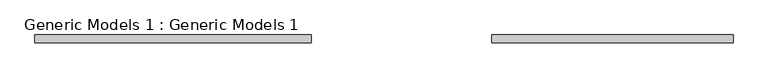
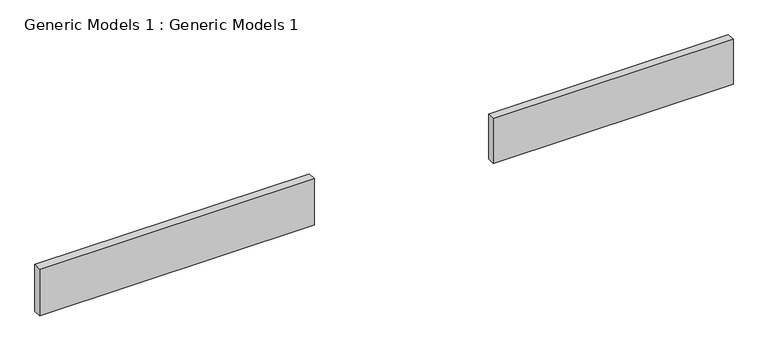
"""IFC4 building model written with IfcOpenShell, lengths in millimetres: proxy geometry, Generic Models 1 : Generic Models 1."""

from ifc_helpers import new_model, si_unit, frame, origin, place, context, project, spatial, polyline, outline, extrude, source, transform, mapped, element, save


def generic_models_1_generic_models_1_e0ba6133(model_context):
    return source(origin(), model_context, "Body", "SweptSolid", [
        extrude(outline(polyline([(5733.7651683, -9812.6503266), (1161.7651683, -9812.6503266), (1161.7651683, -9660.2503266), (5733.7651683, -9660.2503266), (5733.7651683, -9812.6503266)])), frame((0.0, 0.0, 357.9881609), z_axis=(0.0, 0.0, 1.0), x_axis=(1.0, 0.0, 0.0)), (0.0, 0.0, 1.0), 901.097394),
        extrude(outline(polyline([(-2253.6679045, -9812.6503266), (-7486.0679045, -9812.6503266), (-7486.0679045, -9660.2503266), (-2253.6679045, -9660.2503266), (-2253.6679045, -9812.6503266)])), frame((0.0, 0.0, 312.1459104), z_axis=(0.0, 0.0, 1.0), x_axis=(1.0, 0.0, 0.0)), (0.0, 0.0, 1.0), 939.8),
    ])


if __name__ == "__main__":
    model = new_model("IFC4")
    model_context = context("Model", 3, world=origin())
    ifc_project = project(units=[si_unit("LENGTHUNIT", "METRE", prefix="MILLI")], contexts=[model_context])
    site = spatial("IfcSite", under=ifc_project)
    building = spatial("IfcBuilding", under=site)
    placement = place(None, origin())
    generic_models_1_generic_models_1_shape = generic_models_1_generic_models_1_e0ba6133(model_context)
    element("IfcBuildingElementProxy", 1, Name="Generic Models 1 : Generic Models 1", ObjectType="Generic Models 1 : Generic Models 1", at=placement, inside=building, context=model_context, shape_type="MappedRepresentation", body=[
        mapped(generic_models_1_generic_models_1_shape, transform((0.0, 0.0, 0.0), x_axis=(1.0, 0.0, 0.0), y_axis=(0.0, 1.0, 0.0), z_axis=(0.0, 0.0, 1.0))),
    ])
    save(model, "model.ifc")

# Revit data of these elements
# Element 1 (IfcBuildingElementProxy, "Generic Models 1 : Generic Models 1")
#   Materials on its faces: "Parking Stripe"
# Materials
#   "Parking Stripe": class "Paint", colour RGB 250 250 91, transparency 0, Cost = 0
